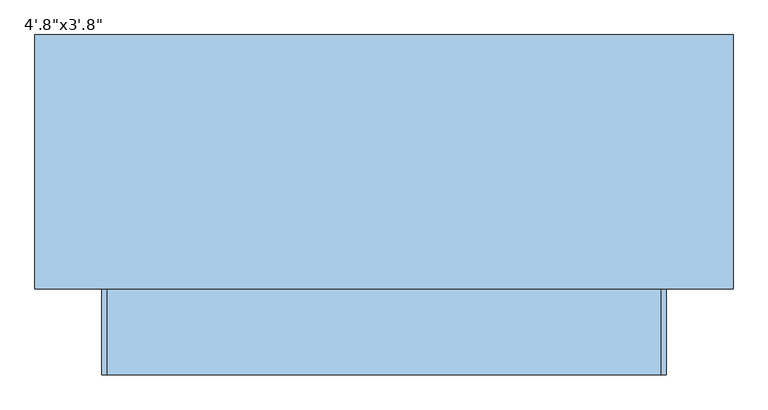
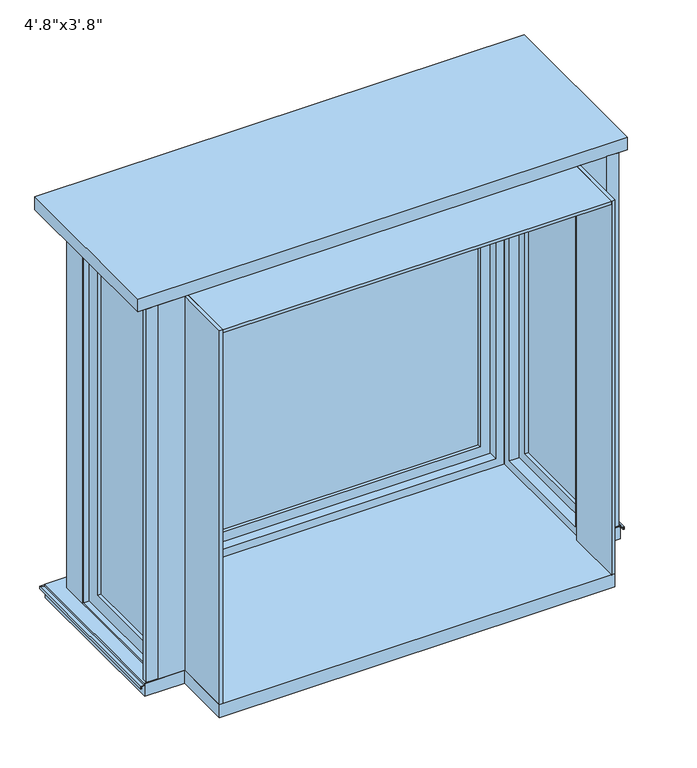
"""IFC4 building model written with IfcOpenShell, lengths in millimetres: window geometry."""

from ifc_helpers import new_model, si_unit, frame, origin, place, context, project, spatial, polyline, outline, extrude, faceted_brep, source, transform, mapped, element, save


def window_19bbd869(model_context):
    return source(origin(), model_context, "Body", "SolidModel", [
        extrude(outline(polyline([(-851.6, 114.3), (-896.05, 114.3), (-896.05, 133.35), (-851.6, 133.35), (-851.6, 114.3)])), frame((0.0, 0.0, 653.5486341), z_axis=(0.0, 0.0, 1.0), x_axis=(1.0, 0.0, 0.0)), (0.0, 0.0, 1.0), 1497.2513659),
        extrude(outline(polyline([(896.05, 114.3), (851.6, 114.3), (851.6, 133.35), (896.05, 133.35), (896.05, 114.3)])), frame((0.0, 0.0, 653.5486341), z_axis=(0.0, 0.0, 1.0), x_axis=(1.0, 0.0, 0.0)), (0.0, 0.0, 1.0), 1497.2513659),
        faceted_brep([(-902.4, 114.3, 643.4697935), (-902.4, 114.3, 650.8), (-851.6, 114.3, 650.8), (-851.6, 114.3, 653.5486341), (-903.797, 114.3, 653.5486341), (-903.797, 114.3, 644.8483503), (-916.497, 114.3, 642.6089977), (-916.497, 114.3, 633.6668038), (-912.5346, 114.3, 633.6668038), (-912.5346, 114.3, 635.1270038), (-914.8968, 114.3, 635.1270038), (-914.8968, 114.3, 641.2662705), (902.4, 114.3, 643.4697935), (914.8968, 114.3, 641.2662705), (914.8968, 114.3, 635.1270038), (912.5346, 114.3, 635.1270038), (912.5346, 114.3, 633.6668038), (916.497, 114.3, 633.6668038), (916.497, 114.3, 642.6089977), (903.797, 114.3, 644.8483503), (903.797, 114.3, 653.5486341), (851.6, 114.3, 653.5486341), (851.6, 114.3, 650.8), (902.4, 114.3, 650.8), (-902.4, 765.1, 643.4697935), (-902.4, 765.1, 650.8), (902.4, 765.1, 650.8), (851.6, 714.3, 650.8), (-851.6, 714.3, 650.8), (-851.6, 714.3, 653.5486341), (851.6, 714.3, 653.5486341), (903.797, 766.497, 653.5486341), (-903.797, 766.497, 653.5486341), (-903.797, 766.497, 644.8483503), (-916.497, 779.197, 642.6089977), (-916.497, 779.197, 633.6668038), (916.497, 779.197, 633.6668038), (912.5346, 775.2346, 633.6668038), (-912.5346, 775.2346, 633.6668038), (-912.5346, 775.2346, 635.1270038), (912.5346, 775.2346, 635.1270038), (914.8968, 777.5968, 635.1270038), (-914.8968, 777.5968, 635.1270038), (-914.8968, 777.5968, 641.2662705), (902.4, 765.1, 643.4697935), (903.797, 766.497, 644.8483503), (916.497, 779.197, 642.6089977), (914.8968, 777.5968, 641.2662705)], [[[0, 1, 2, 3, 4, 5, 6, 7, 8, 9, 10, 11]], [[12, 13, 14, 15, 16, 17, 18, 19, 20, 21, 22, 23]], [[1, 0, 24, 25]], [[2, 1, 25, 26, 23, 22, 27, 28]], [[3, 2, 28, 29]], [[4, 3, 29, 30, 21, 20, 31, 32]], [[5, 4, 32, 33]], [[6, 5, 33, 34]], [[7, 6, 34, 35]], [[8, 7, 35, 36, 17, 16, 37, 38]], [[9, 8, 38, 39]], [[10, 9, 39, 40, 15, 14, 41, 42]], [[11, 10, 42, 43]], [[0, 11, 43, 24]], [[25, 24, 44, 26]], [[29, 28, 27, 30]], [[33, 32, 31, 45]], [[34, 33, 45, 46]], [[35, 34, 46, 36]], [[39, 38, 37, 40]], [[43, 42, 41, 47]], [[24, 43, 47, 44]], [[26, 44, 12, 23]], [[30, 27, 22, 21]], [[45, 31, 20, 19]], [[46, 45, 19, 18]], [[36, 46, 18, 17]], [[40, 37, 16, 15]], [[47, 41, 14, 13]], [[44, 47, 13, 12]]]),
        extrude(outline(polyline([(902.4, 765.1), (902.4, 114.3), (750.0, 114.3), (750.0, -114.3), (-750.0, -114.3), (-750.0, 114.3), (-902.4, 114.3), (-902.4, 765.1), (902.4, 765.1)])), frame((0.0, 0.0, 600.0), z_axis=(0.0, 0.0, 1.0), x_axis=(1.0, 0.0, 0.0)), (0.0, 0.0, 1.0), 50.8),
        extrude(outline(polyline([(927.8, 790.5), (927.8, 114.3), (-927.8, 114.3), (-927.8, 790.5), (927.8, 790.5)])), frame((0.0, 0.0, 2150.8), z_axis=(0.0, 0.0, 1.0), x_axis=(1.0, 0.0, 0.0)), (0.0, 0.0, 1.0), 50.8),
        extrude(outline(polyline([(-750.0, 714.3), (-750.0, 612.7), (-851.6, 612.7), (-851.6, 714.3), (-750.0, 714.3)])), frame((0.0, 0.0, 650.8), z_axis=(0.0, 0.0, 1.0), x_axis=(1.0, 0.0, 0.0)), (0.0, 0.0, 1.0), 1500.0),
        extrude(outline(polyline([(851.6, 714.3), (851.6, 612.7), (750.0, 612.7), (750.0, 714.3), (851.6, 714.3)])), frame((0.0, 0.0, 650.8), z_axis=(0.0, 0.0, 1.0), x_axis=(1.0, 0.0, 0.0)), (0.0, 0.0, 1.0), 1500.0),
        faceted_brep([(737.3, 650.8, 663.5), (737.3, 714.3, 663.5), (-737.3, 714.3, 663.5), (-737.3, 650.8, 663.5), (718.25, 612.7, 682.55), (718.25, 650.8, 682.55), (-718.25, 650.8, 682.55), (-718.25, 612.7, 682.55), (750.0, 714.3, 650.8), (750.0, 612.7, 650.8), (-750.0, 612.7, 650.8), (-750.0, 714.3, 650.8), (-737.3, 714.3, 2138.1), (-737.3, 650.8, 2138.1), (-718.25, 650.8, 2119.05), (-718.25, 612.7, 2119.05), (-750.0, 612.7, 2150.8), (-750.0, 714.3, 2150.8), (737.3, 714.3, 2138.1), (737.3, 650.8, 2138.1), (718.25, 650.8, 2119.05), (718.25, 612.7, 2119.05), (750.0, 612.7, 2150.8), (750.0, 714.3, 2150.8)], [[[0, 1, 2, 3]], [[4, 5, 6, 7]], [[8, 9, 10, 11]], [[3, 2, 12, 13]], [[7, 6, 14, 15]], [[11, 10, 16, 17]], [[13, 12, 18, 19]], [[15, 14, 20, 21]], [[17, 16, 22, 23]], [[11, 17, 23, 8], [1, 18, 12, 2]], [[19, 18, 1, 0]], [[3, 13, 19, 0], [5, 20, 14, 6]], [[21, 20, 5, 4]], [[9, 22, 16, 10], [7, 15, 21, 4]], [[23, 22, 9, 8]]]),
        extrude(outline(polyline([(2138.1, -737.3), (663.5, -737.3), (663.5, 737.3), (2138.1, 737.3), (2138.1, -737.3)]), holes=[polyline([(2080.95, 680.15), (720.65, 680.15), (720.65, -680.15), (2080.95, -680.15), (2080.95, 680.15)])]), frame((0.0, 650.8, 0.0), z_axis=(0.0, 1.0, 0.0), x_axis=(0.0, 0.0, 1.0)), (0.0, 0.0, 1.0), 44.45),
        faceted_brep([(-750.0, 146.05, 2119.05), (-788.1, 146.05, 2119.05), (-788.1, 580.95, 2119.05), (-750.0, 580.95, 2119.05), (-851.6, 114.3, 2150.8), (-750.0, 114.3, 2150.8), (-750.0, 612.7, 2150.8), (-851.6, 612.7, 2150.8), (-788.1, 127.0, 2138.1), (-851.6, 127.0, 2138.1), (-851.6, 600.0, 2138.1), (-788.1, 600.0, 2138.1), (-788.1, 580.95, 682.55), (-750.0, 580.95, 682.55), (-750.0, 612.7, 650.8), (-851.6, 612.7, 650.8), (-851.6, 600.0, 663.5), (-788.1, 600.0, 663.5), (-788.1, 146.05, 682.55), (-750.0, 146.05, 682.55), (-750.0, 114.3, 650.8), (-851.6, 114.3, 650.8), (-851.6, 127.0, 663.5), (-788.1, 127.0, 663.5)], [[[0, 1, 2, 3]], [[4, 5, 6, 7]], [[8, 9, 10, 11]], [[3, 2, 12, 13]], [[7, 6, 14, 15]], [[11, 10, 16, 17]], [[13, 12, 18, 19]], [[15, 14, 20, 21]], [[17, 16, 22, 23]], [[11, 17, 23, 8], [1, 18, 12, 2]], [[19, 18, 1, 0]], [[5, 20, 14, 6], [3, 13, 19, 0]], [[21, 20, 5, 4]], [[7, 15, 21, 4], [9, 22, 16, 10]], [[23, 22, 9, 8]]]),
        extrude(outline(polyline([(600.0, 2138.1), (600.0, 663.5), (127.0, 663.5), (127.0, 2138.1), (600.0, 2138.1)]), holes=[polyline([(184.15, 2080.95), (184.15, 720.65), (542.85, 720.65), (542.85, 2080.95), (184.15, 2080.95)])]), frame((-832.55, 0.0, 0.0), z_axis=(1.0, 0.0, 0.0), x_axis=(0.0, 1.0, 0.0)), (0.0, 0.0, 1.0), 44.45),
        faceted_brep([(788.1, 146.05, 2119.05), (750.0, 146.05, 2119.05), (750.0, 580.95, 2119.05), (788.1, 580.95, 2119.05), (851.6, 127.0, 2138.1), (788.1, 127.0, 2138.1), (788.1, 600.0, 2138.1), (851.6, 600.0, 2138.1), (750.0, 114.3, 2150.8), (851.6, 114.3, 2150.8), (851.6, 612.7, 2150.8), (750.0, 612.7, 2150.8), (750.0, 580.95, 682.55), (788.1, 580.95, 682.55), (788.1, 600.0, 663.5), (851.6, 600.0, 663.5), (851.6, 612.7, 650.8), (750.0, 612.7, 650.8), (750.0, 146.05, 682.55), (788.1, 146.05, 682.55), (788.1, 127.0, 663.5), (851.6, 127.0, 663.5), (851.6, 114.3, 650.8), (750.0, 114.3, 650.8)], [[[0, 1, 2, 3]], [[4, 5, 6, 7]], [[8, 9, 10, 11]], [[3, 2, 12, 13]], [[7, 6, 14, 15]], [[11, 10, 16, 17]], [[13, 12, 18, 19]], [[15, 14, 20, 21]], [[17, 16, 22, 23]], [[11, 17, 23, 8], [1, 18, 12, 2]], [[19, 18, 1, 0]], [[5, 20, 14, 6], [3, 13, 19, 0]], [[21, 20, 5, 4]], [[9, 22, 16, 10], [7, 15, 21, 4]], [[23, 22, 9, 8]]]),
        extrude(outline(polyline([(600.0, 2138.1), (600.0, 663.5), (127.0, 663.5), (127.0, 2138.1), (600.0, 2138.1)]), holes=[polyline([(184.15, 2080.95), (184.15, 720.65), (542.85, 720.65), (542.85, 2080.95), (184.15, 2080.95)])]), frame((788.1, 0.0, 0.0), z_axis=(1.0, 0.0, 0.0), x_axis=(0.0, 1.0, 0.0)), (0.0, 0.0, 1.0), 44.45),
        extrude(outline(polyline([(680.15, 682.55), (680.15, 676.2), (-680.15, 676.2), (-680.15, 682.55), (680.15, 682.55)])), frame((0.0, 0.0, 720.65), z_axis=(0.0, 0.0, 1.0), x_axis=(1.0, 0.0, 0.0)), (0.0, 0.0, 1.0), 1360.3),
        extrude(outline(polyline([(680.15, 669.85), (680.15, 663.5), (-680.15, 663.5), (-680.15, 669.85), (680.15, 669.85)])), frame((0.0, 0.0, 720.65), z_axis=(0.0, 0.0, 1.0), x_axis=(1.0, 0.0, 0.0)), (0.0, 0.0, 1.0), 1360.3),
        extrude(outline(polyline([(-813.5, 542.85), (-813.5, 184.15), (-819.85, 184.15), (-819.85, 542.85), (-813.5, 542.85)])), frame((0.0, 0.0, 720.65), z_axis=(0.0, 0.0, 1.0), x_axis=(1.0, 0.0, 0.0)), (0.0, 0.0, 1.0), 1360.3),
        extrude(outline(polyline([(-800.8, 542.85), (-800.8, 184.15), (-807.15, 184.15), (-807.15, 542.85), (-800.8, 542.85)])), frame((0.0, 0.0, 720.65), z_axis=(0.0, 0.0, 1.0), x_axis=(1.0, 0.0, 0.0)), (0.0, 0.0, 1.0), 1360.3),
        extrude(outline(polyline([(819.85, 542.85), (819.85, 184.15), (813.5, 184.15), (813.5, 542.85), (819.85, 542.85)])), frame((0.0, 0.0, 720.65), z_axis=(0.0, 0.0, 1.0), x_axis=(1.0, 0.0, 0.0)), (0.0, 0.0, 1.0), 1360.3),
        extrude(outline(polyline([(807.15, 542.85), (807.15, 184.15), (800.8, 184.15), (800.8, 542.85), (807.15, 542.85)])), frame((0.0, 0.0, 720.65), z_axis=(0.0, 0.0, 1.0), x_axis=(1.0, 0.0, 0.0)), (0.0, 0.0, 1.0), 1360.3),
        faceted_brep([(851.6, 127.0, 2138.1), (788.1, 127.0, 2138.1), (788.1, 600.0, 2138.1), (851.6, 600.0, 2138.1), (750.0, 114.3, 2150.8), (851.6, 114.3, 2150.8), (851.6, 612.7, 2150.8), (750.0, 612.7, 2150.8), (788.1, 146.05, 2119.05), (750.0, 146.05, 2119.05), (750.0, 580.95, 2119.05), (788.1, 580.95, 2119.05), (788.1, 600.0, 663.5), (851.6, 600.0, 663.5), (851.6, 612.7, 650.8), (750.0, 612.7, 650.8), (750.0, 580.95, 682.55), (788.1, 580.95, 682.55), (788.1, 127.0, 663.5), (851.6, 127.0, 663.5), (851.6, 114.3, 650.8), (750.0, 114.3, 650.8), (750.0, 146.05, 682.55), (788.1, 146.05, 682.55)], [[[0, 1, 2, 3]], [[4, 5, 6, 7]], [[8, 9, 10, 11]], [[3, 2, 12, 13]], [[7, 6, 14, 15]], [[11, 10, 16, 17]], [[13, 12, 18, 19]], [[15, 14, 20, 21]], [[17, 16, 22, 23]], [[1, 18, 12, 2], [11, 17, 23, 8]], [[19, 18, 1, 0]], [[5, 20, 14, 6], [3, 13, 19, 0]], [[21, 20, 5, 4]], [[7, 15, 21, 4], [9, 22, 16, 10]], [[23, 22, 9, 8]]]),
        extrude(outline(polyline([(-737.3, 114.3), (-737.3, -114.3), (-750.0, -114.3), (-750.0, 114.3), (-737.3, 114.3)])), frame((0.0, 0.0, 650.8), z_axis=(0.0, 0.0, 1.0), x_axis=(1.0, 0.0, 0.0)), (0.0, 0.0, 1.0), 1500.0),
        extrude(outline(polyline([(737.3, 114.3), (750.0, 114.3), (750.0, -114.3), (737.3, -114.3), (737.3, 114.3)])), frame((0.0, 0.0, 650.8), z_axis=(0.0, 0.0, 1.0), x_axis=(1.0, 0.0, 0.0)), (0.0, 0.0, 1.0), 1500.0),
        extrude(outline(polyline([(737.3, -114.3), (-737.3, -114.3), (-737.3, 612.7), (737.3, 612.7), (737.3, -114.3)])), frame((0.0, 0.0, 2138.1), z_axis=(0.0, 0.0, 1.0), x_axis=(1.0, 0.0, 0.0)), (0.0, 0.0, 1.0), 12.7),
    ])


if __name__ == "__main__":
    model = new_model("IFC4")
    model_context = context("Model", 3, world=origin())
    ifc_project = project(units=[si_unit("LENGTHUNIT", "METRE", prefix="MILLI")], contexts=[model_context])
    site = spatial("IfcSite", under=ifc_project)
    building = spatial("IfcBuilding", under=site)
    placement = place(None, origin())
    window_shape = window_19bbd869(model_context)
    element("IfcWindow", 1, ObjectType="4'.8\"x3'.8\"", at=placement, inside=building, context=model_context, shape_type="MappedRepresentation", body=[
        mapped(window_shape, transform((0.0, 0.0, 0.0), x_axis=(1.0, 0.0, 0.0), y_axis=(0.0, 1.0, 0.0), z_axis=(0.0, 0.0, 1.0))),
    ])
    save(model, "model.ifc")

# Revit data of these elements
# Type "4'.8\"x3'.8\""
#   Type Mark = "20"
#   Fire Rating = "0.5h"
#   Assembly Code = "B2020100"
#   Analytic Construction = "1/8 in Pilkington single glazing"
#   Width = 4' - 11.05512"
#   Wall Thickness [instance default] = 0' - 5.90551"
#   Visual Light Transmittance = 0.9
#   Trim Width = 5' - 7.05512"
#   Trim Height = 4' - 11.05512"
#   Thermal Resistance (R) = 1.5394 (h·ft²·°F)/BTU
#   Solar Heat Gain Coefficient = 0.86
#   Rough Width = 4' - 11.64567"
#   Rough Height = 4' - 11.64567"
#   Height 1 = 5' - 1.05512"
#   Height = 4' - 11.05512"
#   Heat Transfer Coefficient (U) = 0.6496 BTU/(h·ft²·°F)
#   Depth = 1' - 11.62205"
#   Default Sill Height = 1' - 11.62205"
#   Side Muntin Visibility = yes
#   Center Muntin Visibility = yes
#   Interior Trim Visibility [instance default] = yes
#   Exterior Trim Visibility [instance default] = yes
#   Side Muntin Pattern = M_Muntin Pattern_2x2 : M_Muntin Pattern_2x2
#   Center Muntin Pattern = M_Muntin Pattern_2x2 : M_Muntin Pattern_2x2
#   Interior Trim Material = Wood - Stained
#   Exterior Trim Material = Clad - White
#   Exterior Trim = element 422966
#   Interior Trim = M_Trim-Window-Interior-Flat : Picture Frame
#   Interior Frame Material = Wood - Stained
#   Glass Panel Material = Glass
#   Exterior Frame Material = Clad - White
#   Wall Closure = (empty or 0)
# Element 1 (IfcWindow, "4'.8\"x3'.8\"")
#   Wall Thickness = 0' - 9"
#   Materials on its faces: "Clad - White", "Wood - Stained", "Glass"
# Materials
#   "Wood - Stained": class "Wood", colour RGB 224 178 126, transparency 0, Cost = 0
#   "Clad - White": class "Wood", colour RGB 242 242 238, transparency 0, Cost = 0
#   "Glass": class "Glass", colour RGB 0 128 192, transparency 0.75, Description = "Soda Lime Glass", Cost = 0
